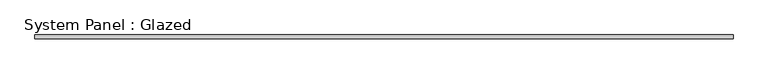
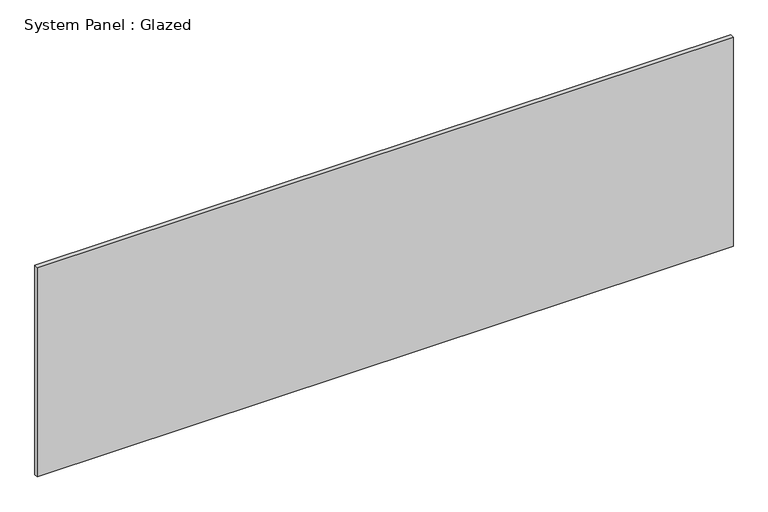
"""IFC4 building model written with IfcOpenShell, lengths in millimetres: plate geometry, System Panel : Glazed."""

from ifc_helpers import new_model, si_unit, origin, origin_with_axes, place, context, project, spatial, polyline, outline, extrude, source, transform, mapped, element, save


def system_panel_glazed_7f285cc4(model_context):
    return source(origin(), model_context, "Body", "SweptSolid", [
        extrude(outline(polyline([(2298.7, 19.05), (-2298.7, 19.05), (-2298.7, 44.45), (2298.7, 44.45), (2298.7, 19.05)])), origin_with_axes(), (0.0, 0.0, 1.0), 1460.5),
    ])


if __name__ == "__main__":
    model = new_model("IFC4")
    model_context = context("Model", 3, world=origin())
    ifc_project = project(units=[si_unit("LENGTHUNIT", "METRE", prefix="MILLI")], contexts=[model_context])
    site = spatial("IfcSite", under=ifc_project)
    building = spatial("IfcBuilding", under=site)
    placement = place(None, origin())
    system_panel_glazed_shape = system_panel_glazed_7f285cc4(model_context)
    element("IfcPlate", 1, ObjectType="System Panel : Glazed", at=placement, inside=building, context=model_context, shape_type="MappedRepresentation", body=[
        mapped(system_panel_glazed_shape, transform((0.0, 0.0, 0.0), x_axis=(1.0, 0.0, 0.0), y_axis=(0.0, 1.0, 0.0), z_axis=(0.0, 0.0, 1.0))),
    ])
    save(model, "model.ifc")

# Revit data of these elements
# Type "System Panel : Glazed"
#   Construction Type Id = "GSP4R"
#   Analytic Construction = "1/8 in Pilkington single glazing"
#   Visual Light Transmittance = 0.9
#   Solar Heat Gain Coefficient = 0.86
#   Heat Transfer Coefficient (U) = 1.18115 BTU/(h·ft²·°F)
# Element 1 (IfcPlate, "System Panel : Glazed")
#   Materials on its faces: "Glass"
# Materials
#   "Glass": class "Glass", colour RGB 0 128 192, transparency 0.75, Description = "Soda Lime Glass", Cost = 0
